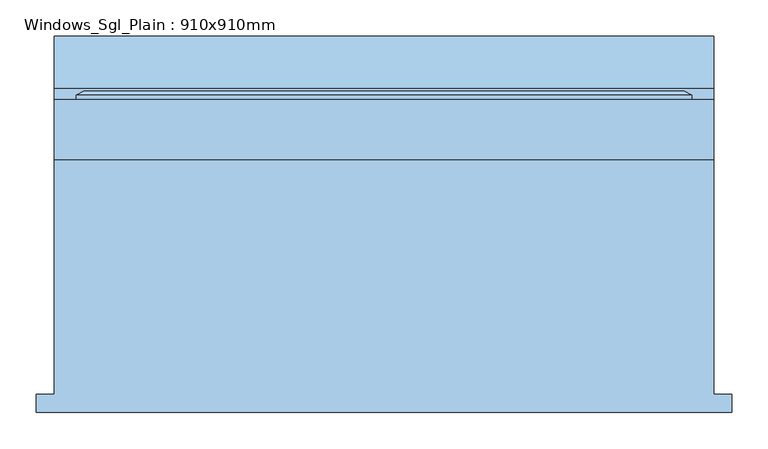
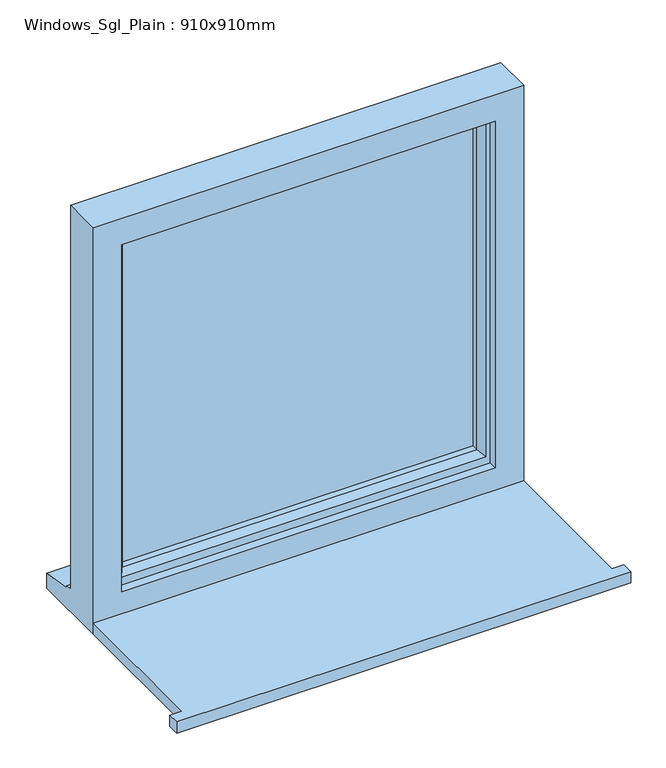
"""IFC4 building model written with IfcOpenShell, lengths in millimetres: window geometry, Windows_Sgl_Plain : 910x910mm."""

from ifc_helpers import new_model, si_unit, frame, origin, place, context, project, spatial, polyline, outline, extrude, faceted_brep, source, transform, mapped, element, save


def windows_sgl_plain_910x910mm_4715da24(model_context):
    return source(origin(), model_context, "Body", "SolidModel", [
        extrude(outline(polyline([(-480.0, -245.1434322), (-480.0, -220.1434322), (-455.0, -220.1434322), (-455.0, 104.0565678), (455.0, 104.0565678), (455.0, -220.1434322), (480.0, -220.1434322), (480.0, -245.1434322), (-480.0, -245.1434322)])), frame((0.0, 0.0, 1200.0), z_axis=(0.0, 0.0, 1.0), x_axis=(1.0, 0.0, 0.0)), (0.0, 0.0, 1.0), 25.0),
        faceted_brep([(-455.0, 104.0565678, 1200.0), (455.0, 104.0565678, 1200.0), (455.0, 104.0565678, 2110.0), (-455.0, 104.0565678, 2110.0), (-395.0, 104.0565678, 2050.0), (395.0, 104.0565678, 2050.0), (395.0, 104.0565678, 1275.0), (-395.0, 104.0565678, 1275.0), (-455.0, 187.0565678, 2110.0), (-455.0, 187.0565678, 1251.0), (-455.0, 202.0565678, 1249.68767), (-455.0, 202.0565678, 1244.7449676), (-455.0, 274.5565678, 1233.8088847), (-455.0, 274.5565678, 1200.0), (455.0, 187.0565678, 2110.0), (455.0, 187.0565678, 1251.0), (-415.0, 187.0565678, 2070.0), (-415.0, 187.0565678, 1263.0), (415.0, 187.0565678, 1263.0), (415.0, 187.0565678, 2070.0), (-415.0, 122.0565678, 2070.0), (-415.0, 122.0565678, 1263.0), (415.0, 122.0565678, 2070.0), (415.0, 122.0565678, 1263.0), (-395.0, 122.0565678, 2050.0), (-395.0, 122.0565678, 1275.0), (395.0, 122.0565678, 1275.0), (395.0, 122.0565678, 2050.0), (455.0, 274.5565678, 1200.0), (455.0, 274.5565678, 1233.8088847), (455.0, 202.0565678, 1244.7449676), (455.0, 202.0565678, 1249.68767)], [[[0, 1, 2, 3], [4, 5, 6, 7]], [[0, 3, 8, 9, 10, 11, 12, 13]], [[9, 8, 14, 15], [16, 17, 18, 19]], [[17, 16, 20, 21]], [[20, 22, 23, 21], [24, 25, 26, 27]], [[24, 4, 7, 25]], [[3, 2, 14, 8]], [[16, 19, 22, 20]], [[5, 4, 24, 27]], [[15, 14, 2, 1, 28, 29, 30, 31]], [[19, 18, 23, 22]], [[5, 27, 26, 6]], [[28, 1, 0, 13]], [[29, 28, 13, 12]], [[30, 29, 12, 11]], [[31, 30, 11, 10]], [[15, 31, 10, 9]], [[21, 23, 18, 17]], [[7, 6, 26, 25]]]),
        extrude(outline(polyline([(385.0, 151.0565678), (-385.0, 151.0565678), (-385.0, 175.0565678), (385.0, 175.0565678), (385.0, 151.0565678)])), frame((0.0, 0.0, 1293.0), z_axis=(0.0, 0.0, 1.0), x_axis=(1.0, 0.0, 0.0)), (0.0, 0.0, 1.0), 747.0),
        faceted_brep([(-425.0, 187.0565678, 2080.0), (-425.0, 192.8300705, 2080.0), (-425.0, 192.8300705, 1253.0), (-425.0, 187.0565678, 1253.0), (-415.0, 122.0565678, 2070.0), (-415.0, 187.0565678, 2070.0), (-415.0, 187.0565678, 1263.0), (-415.0, 122.0565678, 1263.0), (-375.0, 136.5494677, 2030.0), (-385.1480377, 122.0565678, 2040.1480377), (-385.1480377, 122.0565678, 1292.8519623), (-375.0, 136.5494677, 1303.0), (-375.0, 151.0565678, 2030.0), (-375.0, 151.0565678, 1303.0), (-385.0, 175.0565678, 2040.0), (-385.0, 151.0565678, 2040.0), (-385.0, 151.0565678, 1293.0), (-385.0, 175.0565678, 1293.0), (-375.0, 192.8300705, 2030.0), (-375.0, 175.0565678, 2030.0), (-375.0, 175.0565678, 1303.0), (-375.0, 192.8300705, 1303.0), (-392.4457548, 198.6035732, 2047.4457548), (-392.4457548, 198.6035732, 1285.5542452), (-414.2153903, 198.6035732, 2069.2153903), (-414.2153903, 198.6035732, 1263.7846097), (425.0, 192.8300705, 1253.0), (425.0, 187.0565678, 1253.0), (415.0, 187.0565678, 1263.0), (415.0, 122.0565678, 1263.0), (385.1480377, 122.0565678, 1292.8519623), (375.0, 136.5494677, 1303.0), (375.0, 151.0565678, 1303.0), (385.0, 151.0565678, 1293.0), (385.0, 175.0565678, 1293.0), (375.0, 175.0565678, 1303.0), (375.0, 192.8300705, 1303.0), (392.4457548, 198.6035732, 1285.5542452), (414.2153903, 198.6035732, 1263.7846097), (425.0, 192.8300705, 2080.0), (425.0, 187.0565678, 2080.0), (415.0, 187.0565678, 2070.0), (415.0, 122.0565678, 2070.0), (385.1480377, 122.0565678, 2040.1480377), (375.0, 136.5494677, 2030.0), (375.0, 151.0565678, 2030.0), (385.0, 151.0565678, 2040.0), (385.0, 175.0565678, 2040.0), (375.0, 175.0565678, 2030.0), (375.0, 192.8300705, 2030.0), (392.4457548, 198.6035732, 2047.4457548), (414.2153903, 198.6035732, 2069.2153903)], [[[0, 1, 2, 3]], [[4, 5, 6, 7]], [[8, 9, 10, 11]], [[12, 8, 11, 13]], [[14, 15, 16, 17]], [[18, 19, 20, 21]], [[22, 18, 21, 23]], [[1, 24, 25, 2]], [[3, 2, 26, 27]], [[7, 6, 28, 29]], [[11, 10, 30, 31]], [[13, 11, 31, 32]], [[17, 16, 33, 34]], [[21, 20, 35, 36]], [[23, 21, 36, 37]], [[2, 25, 38, 26]], [[27, 26, 39, 40]], [[29, 28, 41, 42]], [[31, 30, 43, 44]], [[32, 31, 44, 45]], [[34, 33, 46, 47]], [[36, 35, 48, 49]], [[37, 36, 49, 50]], [[26, 38, 51, 39]], [[40, 39, 1, 0]], [[3, 27, 40, 0], [5, 41, 28, 6]], [[42, 41, 5, 4]], [[7, 29, 42, 4], [9, 43, 30, 10]], [[44, 43, 9, 8]], [[45, 44, 8, 12]], [[15, 46, 33, 16], [13, 32, 45, 12]], [[47, 46, 15, 14]], [[17, 34, 47, 14], [19, 48, 35, 20]], [[49, 48, 19, 18]], [[50, 49, 18, 22]], [[24, 51, 38, 25], [23, 37, 50, 22]], [[39, 51, 24, 1]]]),
    ])


if __name__ == "__main__":
    model = new_model("IFC4")
    model_context = context("Model", 3, world=origin())
    ifc_project = project(units=[si_unit("LENGTHUNIT", "METRE", prefix="MILLI")], contexts=[model_context])
    site = spatial("IfcSite", under=ifc_project)
    building = spatial("IfcBuilding", under=site)
    placement = place(None, origin())
    windows_sgl_plain_910x910mm_shape = windows_sgl_plain_910x910mm_4715da24(model_context)
    element("IfcWindow", 1, ObjectType="Windows_Sgl_Plain : 910x910mm", at=placement, inside=building, context=model_context, shape_type="MappedRepresentation", body=[
        mapped(windows_sgl_plain_910x910mm_shape, transform((0.0, 0.0, 0.0), x_axis=(1.0, 0.0, 0.0), y_axis=(0.0, 1.0, 0.0), z_axis=(0.0, 0.0, 1.0))),
    ])
    save(model, "model.ifc")

# Revit data of these elements
# Type "Windows_Sgl_Plain : 910x910mm"
#   Type Mark = "44"
#   Operation = "SinglePanel"
#   Construction Type Id = "SGL"
#   Manufacturer = "Revit"
#   Keynote = "L10"
#   Analytic Construction = "Large single-glazed windows"
#   Wrap Layers (Ext) from Ext = 102.5 mm
#   Wrap Layers (Int) from Ext = 177.5 mm
#   Window Board Projection = 25 mm
#   Window Board Extension = 25 mm
#   Visual Light Transmittance = 0.9
#   Solar Heat Gain Coefficient = 0.86
#   Rough Width = 910 mm
#   Rough Height = 910 mm
#   Height = 910 mm
#   Width = 910 mm
#   Heat Transfer Coefficient (U) = 5.5617 W/(m²·K)
#   Glazing Thickness = 24 mm
#   FrameOffset - External = 50 mm
#   Frame Depth = 65 mm
#   Default Head Height = 2110 mm
#   Cill Depth = 87.5 mm
#   Cavity Closer Width = 50 mm
#   Cavity Closer Offset from Ext = 102.5 mm
#   Cavity Closer Depth = 85 mm
#   Define Thermal Properties by = 1
#   Vis - Cavity Closers = yes
#   Define Thermal Properties by = 1
#   Material Trim = Window Frame
#   Material Glass = Glass
#   Material Frame = Window Frame
#   Wall Closure = (empty or 0)
# Element 1 (IfcWindow, "Windows_Sgl_Plain : 910x910mm")
#   Materials on its faces: "Window Frame", "Glass"
# Materials
#   "Window Frame": colour RGB 249 249 249, transparency 0, Keynote = "L10", Cost = 0
#   "Glass": class "Glass", colour RGB 0 128 192, transparency 0.9, Description = "Soda Lime Glass", Cost = 0
